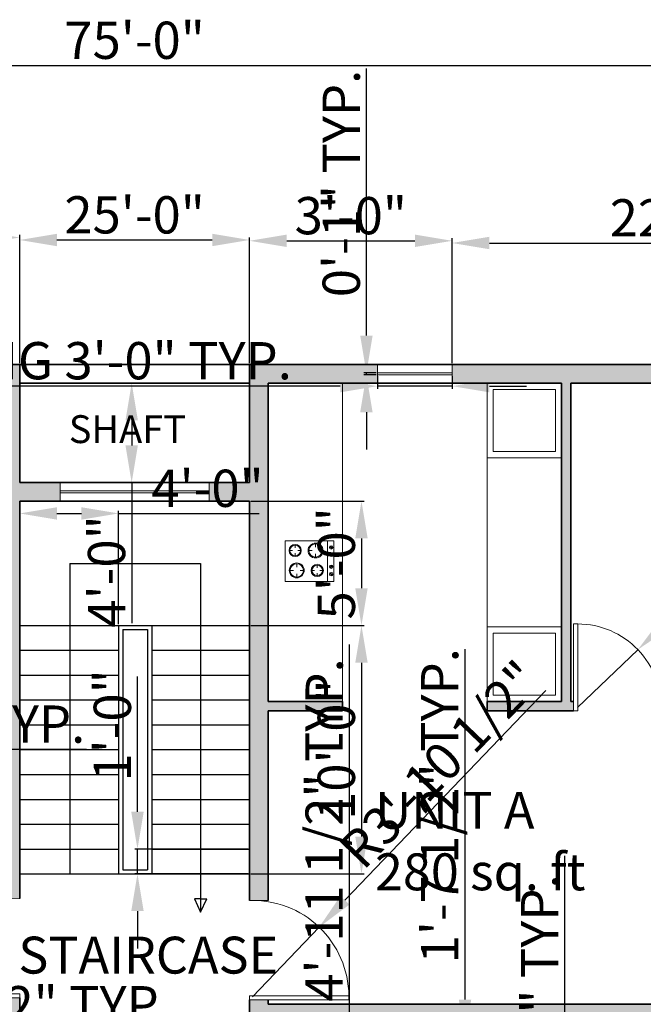
# Model space of a CAD drawing. Units: inches. Extents: x 2043 to 3177, y 1429 to 2563.
# Tile 13 of 14: x 2552 to 2853, y 1952 to 2428. Entities that reach past the tile are written whole.
import ezdxf

# ---------------------------------------------------------------- set-up
doc = ezdxf.new("R2010")
doc.units = ezdxf.units.IN
for name, color, linetype, lineweight in [('A-ANNO-DIMS', 2, 'Continuous', 13), ('A-AREA-IDEN', 7, 'Continuous', 18), ('A-DOOR', 3, 'Continuous', 18), ('A-EQPM', 8, 'Continuous', 18), ('A-FLOR-CASE', 8, 'Continuous', 18), ('A-FLOR-STRS', 7, 'Continuous', 25), ('A-GLAZ', 4, 'Continuous', 18), ('A-WALL', 7, 'Continuous', 35)]:
    doc.layers.add(name, color=color, linetype=linetype, lineweight=lineweight)
doc.layers.add('A-WALL-PATT', color=251, linetype='Continuous', lineweight=13, true_color=0x636466)
doc.styles.get("Standard").update_dxf_attribs({"font": 'arial.ttf'})
doc.dimstyles.new('ISO-25', dxfattribs={"dimtxt": 18, "dimasz": 18, "dimexe": 1.25, "dimexo": 0.625, "dimtad": 1, "dimlunit": 3, "dimtxsty": 'Standard', "dimcen": 2.5, "dimadec": 0, "dimazin": 0, "dimtfac": 1, "dimtmove": 0, "dimatfit": 3, "dimfxl": 1, "dimarcsym": 0})

# ---------------------------------------------------------------- blocks, each defined once
blk = doc.blocks.new('A$C16A60262')
at = {"linetype": 'ByBlock'}
for p, q in [((0, 600), (0, 0)), ((488, 600), (0, 600)), ((0, 600), (500, 600)), ((0, 600), (500, 600)), ((500, 520), (0, 520)), ((500, 600), (500, 0)), ((500, 600), (500, 0)), ((38, 374), (79, 374)), ((119, 456), (119, 415)), ((201, 374), (160, 374)), ((298, 395), (331, 395)), ((363, 460), (363, 427)), ((428, 395), (396, 395)), ((119, 293), (119, 334)), ((363, 330), (363, 362)), ((54, 124), (87, 124)), ((119, 189), (119, 156)), ((184, 124), (152, 124)), ((282, 144), (323, 144)), ((363, 225), (363, 185)), ((445, 144), (404, 144)), ((0, 0), (500, 0)), ((119, 59), (119, 91)), ((363, 63), (363, 103))]:
    blk.add_line(p, q, dxfattribs=at)
for p, q in [((66, 557), (87, 579)), ((72, 552), (66, 557)), ((93, 573), (72, 552)), ((87, 579), (93, 573)), ((158, 572), (163, 578)), ((179, 551), (158, 572)), ((163, 578), (184, 557)), ((184, 557), (179, 551)), ((305, 572), (311, 578)), ((326, 551), (305, 572)), ((311, 578), (332, 557)), ((332, 557), (326, 551)), ((396, 558), (417, 580)), ((402, 553), (396, 558)), ((423, 574), (402, 553)), ((417, 580), (423, 574))]:
    blk.add_line(p, q)
for centre in [(80, 566), (171, 566), (318, 566), (409, 566)]:
    blk.add_circle(centre, 20.6)
for centre, radius in [((119, 374), 91.3), ((119, 374), 81.3), ((363, 395), 75), ((363, 395), 65), ((119, 124), 75), ((119, 124), 65), ((363, 144), 91.3), ((363, 144), 81.3)]:
    blk.add_circle(centre, radius, dxfattribs=at)
blk = doc.blocks.new('*D13')
at = {"layer": 'A-ANNO-DIMS', "color": 0, "lineweight": -2, "transparency": 16777216}
for p, q in [((2453.87, 2262.02), (2453.87, 2324.03)), ((2471.87, 2322.78), (2533.74, 2322.78)), ((2551.74, 2262.02), (2551.74, 2324.03))]:
    blk.add_line(p, q, dxfattribs=at)
at = {"layer": 'A-ANNO-DIMS', "color": 0, "transparency": 16777216}
for points in [[(2471.87, 2325.78), (2471.87, 2319.78), (2453.87, 2322.78)], [(2533.74, 2325.78), (2533.74, 2319.78), (2551.74, 2322.78)]]:
    blk.add_solid(points, dxfattribs=at)
at = {"layer": 'Defpoints', "color": 0, "transparency": 16777216}
for p in [(2551.74, 2322.78), (2453.87, 2261.39), (2551.74, 2261.39)]:
    blk.add_point(p, dxfattribs=at)
at = {"layer": 'A-ANNO-DIMS', "color": 0, "transparency": 16777216, "insert": (2502.81, 2332.6), "char_height": 18, "attachment_point": 5}
blk.add_mtext('3\'-0"', dxfattribs=at)
blk = doc.blocks.new('*D14')
at = {"layer": 'A-ANNO-DIMS', "color": 0, "lineweight": -2, "transparency": 16777216}
for p, q in [((2551.74, 2262.02), (2551.74, 2322.83)), ((2569.74, 2321.58), (2644.74, 2321.58)), ((2662.74, 2262.02), (2662.74, 2322.83))]:
    blk.add_line(p, q, dxfattribs=at)
at = {"layer": 'A-ANNO-DIMS', "color": 0, "transparency": 16777216}
for points in [[(2569.74, 2324.58), (2569.74, 2318.58), (2551.74, 2321.58)], [(2644.74, 2324.58), (2644.74, 2318.58), (2662.74, 2321.58)]]:
    blk.add_solid(points, dxfattribs=at)
at = {"layer": 'Defpoints', "color": 0, "transparency": 16777216}
for p in [(2662.74, 2321.58), (2551.74, 2261.39), (2662.74, 2261.39)]:
    blk.add_point(p, dxfattribs=at)
at = {"layer": 'A-ANNO-DIMS', "color": 0, "transparency": 16777216, "insert": (2607.24, 2331.39), "char_height": 18, "attachment_point": 5}
blk.add_mtext('25\'-0"', dxfattribs=at)
blk = doc.blocks.new('*D15')
at = {"layer": 'A-ANNO-DIMS', "color": 0, "lineweight": -2, "transparency": 16777216}
for p, q in [((2662.74, 2262.02), (2662.74, 2322.43)), ((2680.74, 2321.18), (2742.62, 2321.18)), ((2760.62, 2262.02), (2760.62, 2322.43))]:
    blk.add_line(p, q, dxfattribs=at)
at = {"layer": 'A-ANNO-DIMS', "color": 0, "transparency": 16777216}
for points in [[(2680.74, 2324.18), (2680.74, 2318.18), (2662.74, 2321.18)], [(2742.62, 2324.18), (2742.62, 2318.18), (2760.62, 2321.18)]]:
    blk.add_solid(points, dxfattribs=at)
at = {"layer": 'Defpoints', "color": 0, "transparency": 16777216}
for p in [(2760.62, 2321.18), (2662.74, 2261.39), (2760.62, 2261.39)]:
    blk.add_point(p, dxfattribs=at)
at = {"layer": 'A-ANNO-DIMS', "color": 0, "transparency": 16777216, "insert": (2711.68, 2331), "char_height": 18, "attachment_point": 5}
blk.add_mtext('3\'-0"', dxfattribs=at)
blk = doc.blocks.new('*D16')
at = {"layer": 'A-ANNO-DIMS', "color": 0, "lineweight": -2, "transparency": 16777216}
for p, q in [((2760.62, 2262.02), (2760.62, 2321.37)), ((2980.74, 2262.02), (2980.74, 2321.37)), ((2778.62, 2320.12), (2962.74, 2320.12))]:
    blk.add_line(p, q, dxfattribs=at)
at = {"layer": 'A-ANNO-DIMS', "color": 0, "transparency": 16777216}
for points in [[(2778.62, 2323.12), (2778.62, 2317.12), (2760.62, 2320.12)], [(2962.74, 2323.12), (2962.74, 2317.12), (2980.74, 2320.12)]]:
    blk.add_solid(points, dxfattribs=at)
at = {"layer": 'Defpoints', "color": 0, "transparency": 16777216}
for p in [(2980.74, 2320.12), (2760.62, 2261.39), (2980.74, 2261.39)]:
    blk.add_point(p, dxfattribs=at)
at = {"layer": 'A-ANNO-DIMS', "color": 0, "transparency": 16777216, "insert": (2870.68, 2329.94), "char_height": 18, "attachment_point": 5}
blk.add_mtext('22\'-0"', dxfattribs=at)
blk = doc.blocks.new('*D30')
at = {"layer": 'A-ANNO-DIMS', "color": 0, "lineweight": -2, "transparency": 16777216}
for p, q in [((2233.74, 2262.02), (2233.74, 2407.15)), ((2980.74, 2262.02), (2980.74, 2407.15)), ((2251.74, 2405.9), (2962.74, 2405.9))]:
    blk.add_line(p, q, dxfattribs=at)
at = {"layer": 'A-ANNO-DIMS', "color": 0, "transparency": 16777216}
for points in [[(2251.74, 2408.9), (2251.74, 2402.9), (2233.74, 2405.9)], [(2962.74, 2408.9), (2962.74, 2402.9), (2980.74, 2405.9)]]:
    blk.add_solid(points, dxfattribs=at)
at = {"layer": 'Defpoints', "color": 0, "transparency": 16777216}
for p in [(2980.74, 2405.9), (2233.74, 2261.39), (2980.74, 2261.39)]:
    blk.add_point(p, dxfattribs=at)
at = {"layer": 'A-ANNO-DIMS', "color": 0, "transparency": 16777216, "insert": (2607.24, 2415.72), "char_height": 18, "attachment_point": 5}
blk.add_mtext('75\'-0"', dxfattribs=at)
blk = doc.blocks.new('CASEWORK-TWIN-END-BAYS')
for p, q in [((36, 153.75), (36, 0)), ((3, 150.75), (3, 120.75)), ((3, 150.75), (33, 150.75)), ((33, 150.75), (33, 120.75)), ((3, 120.75), (33, 120.75)), ((0, 117.75), (36, 117.75)), ((0, 36), (36, 36)), ((3, 33), (33, 33)), ((3, 33), (3, 3)), ((33, 33), (33, 3)), ((3, 3), (33, 3))]:
    blk.add_line(p, q)
blk = doc.blocks.new('GLAZING-36')
for p, q in [((0, 36), (0, 0)), ((1, 36), (1, 0))]:
    blk.add_line(p, q)
blk = doc.blocks.new('GLAZING-72')
for p, q in [((72, 1), (0, 1)), ((72, 0), (0, 0))]:
    blk.add_line(p, q)
blk = doc.blocks.new('*D41')
at = {"layer": 'A-ANNO-DIMS', "color": 0, "lineweight": -2, "transparency": 16777216}
for p, q in [((2711.06, 1791.23), (2711.06, 2126.25)), ((2702.73, 1791.23), (2712.31, 1791.23)), ((2711.06, 1749.52), (2711.06, 1773.23)), ((2702.73, 1731.52), (2712.31, 1731.52))]:
    blk.add_line(p, q, dxfattribs=at)
at = {"layer": 'A-ANNO-DIMS', "color": 0, "transparency": 16777216}
for points in [[(2708.06, 1773.23), (2714.06, 1773.23), (2711.06, 1791.23)], [(2708.06, 1749.52), (2714.06, 1749.52), (2711.06, 1731.52)]]:
    blk.add_solid(points, dxfattribs=at)
at = {"layer": 'Defpoints', "color": 0, "transparency": 16777216}
for p in [(2702.11, 1791.23), (2711.06, 1791.23), (2702.11, 1731.52)]:
    blk.add_point(p, dxfattribs=at)
at = {"layer": 'A-ANNO-DIMS', "color": 0, "transparency": 16777216, "insert": (2701.13, 1967.74), "char_height": 18, "attachment_point": 5, "rotation": 90}
blk.add_mtext('LOW TABLE 4\'-11 1/2" TYP.', dxfattribs=at)
blk = doc.blocks.new('*D49')
at = {"layer": 'A-ANNO-DIMS', "color": 0, "lineweight": -2, "transparency": 16777216}
for p, q in [((2724.62, 2255.77), (2724.62, 2249.74)), ((2760.62, 2255.77), (2760.62, 2249.74)), ((2706.62, 2250.99), (2460.58, 2250.99)), ((2760.62, 2250.99), (2724.62, 2250.99)), ((2778.62, 2250.99), (2796.62, 2250.99))]:
    blk.add_line(p, q, dxfattribs=at)
at = {"layer": 'A-ANNO-DIMS', "color": 0, "transparency": 16777216}
for points in [[(2706.62, 2253.99), (2706.62, 2247.99), (2724.62, 2250.99)], [(2778.62, 2253.99), (2778.62, 2247.99), (2760.62, 2250.99)]]:
    blk.add_solid(points, dxfattribs=at)
at = {"layer": 'Defpoints', "color": 0, "transparency": 16777216}
for p in [(2724.62, 2256.39), (2760.62, 2256.39), (2724.62, 2250.99)]:
    blk.add_point(p, dxfattribs=at)
at = {"layer": 'A-ANNO-DIMS', "color": 0, "transparency": 16777216, "insert": (2574.6, 2260.93), "char_height": 18, "attachment_point": 5}
blk.add_mtext('GLAZING 3\'-0" TYP.', dxfattribs=at)
blk = doc.blocks.new('*D50')
at = {"layer": 'A-ANNO-DIMS', "color": 0, "lineweight": -2, "transparency": 16777216}
for p, q in [((2719.22, 2275.39), (2719.22, 2404.36)), ((2723.99, 2257.39), (2717.97, 2257.39)), ((2723.99, 2256.39), (2717.97, 2256.39)), ((2719.22, 2256.39), (2719.22, 2257.39)), ((2719.22, 2238.39), (2719.22, 2220.39))]:
    blk.add_line(p, q, dxfattribs=at)
at = {"layer": 'A-ANNO-DIMS', "color": 0, "transparency": 16777216}
for points in [[(2716.22, 2275.39), (2722.22, 2275.39), (2719.22, 2257.39)], [(2716.22, 2238.39), (2722.22, 2238.39), (2719.22, 2256.39)]]:
    blk.add_solid(points, dxfattribs=at)
at = {"layer": 'Defpoints', "color": 0, "transparency": 16777216}
for p in [(2719.22, 2257.39), (2724.62, 2257.39), (2724.62, 2256.39)]:
    blk.add_point(p, dxfattribs=at)
at = {"layer": 'A-ANNO-DIMS', "color": 0, "transparency": 16777216, "insert": (2709.4, 2348.88), "char_height": 18, "attachment_point": 5, "rotation": 90}
blk.add_mtext('0\'-1" TYP.', dxfattribs=at)
blk = doc.blocks.new('*D57')
at = {"layer": 'A-ANNO-DIMS', "color": 0, "lineweight": -2, "transparency": 16777216}
for p, q in [((2309.03, 1935.24), (2309.03, 1941.18)), ((2344.46, 1935.24), (2344.46, 1941.18)), ((2291.03, 1939.93), (2273.03, 1939.93)), ((2309.03, 1939.93), (2344.46, 1939.93)), ((2362.46, 1939.93), (2629.01, 1939.93))]:
    blk.add_line(p, q, dxfattribs=at)
at = {"layer": 'A-ANNO-DIMS', "color": 0, "transparency": 16777216}
for points in [[(2291.03, 1942.93), (2291.03, 1936.93), (2309.03, 1939.93)], [(2362.46, 1942.93), (2362.46, 1936.93), (2344.46, 1939.93)]]:
    blk.add_solid(points, dxfattribs=at)
at = {"layer": 'Defpoints', "color": 0, "transparency": 16777216}
for p in [(2344.46, 1939.93), (2309.03, 1934.62), (2344.46, 1934.62)]:
    blk.add_point(p, dxfattribs=at)
at = {"layer": 'A-ANNO-DIMS', "color": 0, "transparency": 16777216, "insert": (2504.74, 1949.86), "char_height": 18, "attachment_point": 5}
blk.add_mtext('BASIN 2\'-11 1/2" TYP.', dxfattribs=at)
blk = doc.blocks.new('*D61')
at = {"layer": 'A-ANNO-DIMS', "color": 0, "lineweight": -2, "transparency": 16777216}
for p, q in [((2752.39, 1913.46), (2434.98, 1913.46)), ((2770.39, 1916.38), (2770.39, 1912.21)), ((2794.01, 1913.46), (2770.39, 1913.46)), ((2794.01, 1916.38), (2794.01, 1912.21)), ((2812.01, 1913.46), (2830.01, 1913.46))]:
    blk.add_line(p, q, dxfattribs=at)
at = {"layer": 'A-ANNO-DIMS', "color": 0, "transparency": 16777216}
for points in [[(2752.39, 1916.46), (2752.39, 1910.46), (2770.39, 1913.46)], [(2812.01, 1916.46), (2812.01, 1910.46), (2794.01, 1913.46)]]:
    blk.add_solid(points, dxfattribs=at)
at = {"layer": 'Defpoints', "color": 0, "transparency": 16777216}
for p in [(2770.39, 1917.01), (2794.01, 1917.01), (2770.39, 1913.46)]:
    blk.add_point(p, dxfattribs=at)
at = {"layer": 'A-ANNO-DIMS', "color": 0, "transparency": 16777216, "insert": (2584.68, 1923.4), "char_height": 18, "attachment_point": 5}
blk.add_mtext('COOKTOP 1\'-11 1/2" TYP.', dxfattribs=at)
blk = doc.blocks.new('*D62')
at = {"layer": 'A-ANNO-DIMS', "color": 0, "lineweight": -2, "transparency": 16777216}
for p, q in [((2766.85, 1954.69), (2766.85, 2123.91)), ((2769.77, 1936.69), (2765.6, 1936.69)), ((2766.85, 1917.01), (2766.85, 1936.69)), ((2769.77, 1917.01), (2765.6, 1917.01)), ((2766.85, 1899.01), (2766.85, 1881.01))]:
    blk.add_line(p, q, dxfattribs=at)
at = {"layer": 'A-ANNO-DIMS', "color": 0, "transparency": 16777216}
for points in [[(2763.85, 1954.69), (2769.85, 1954.69), (2766.85, 1936.69)], [(2763.85, 1899.01), (2769.85, 1899.01), (2766.85, 1917.01)]]:
    blk.add_solid(points, dxfattribs=at)
at = {"layer": 'Defpoints', "color": 0, "transparency": 16777216}
for p in [(2766.85, 1936.69), (2770.39, 1936.69), (2770.39, 1917.01)]:
    blk.add_point(p, dxfattribs=at)
at = {"layer": 'A-ANNO-DIMS', "color": 0, "transparency": 16777216, "insert": (2756.92, 2048.3), "char_height": 18, "attachment_point": 5, "rotation": 90}
blk.add_mtext('1\'-7 1/2" TYP.', dxfattribs=at)
blk = doc.blocks.new('*D64')
at = {"layer": 'A-ANNO-DIMS', "color": 0, "lineweight": -2, "transparency": 16777216}
for p, q in [((2400.99, 2098.02), (2400.99, 2074.33)), ((2436.99, 2098.02), (2436.99, 2074.33)), ((2382.99, 2075.58), (2364.99, 2075.58)), ((2400.99, 2075.58), (2436.99, 2075.58)), ((2454.99, 2075.58), (2583.95, 2075.58))]:
    blk.add_line(p, q, dxfattribs=at)
at = {"layer": 'A-ANNO-DIMS', "color": 0, "transparency": 16777216}
for points in [[(2382.99, 2078.58), (2382.99, 2072.58), (2400.99, 2075.58)], [(2454.99, 2078.58), (2454.99, 2072.58), (2436.99, 2075.58)]]:
    blk.add_solid(points, dxfattribs=at)
at = {"layer": 'Defpoints', "color": 0, "transparency": 16777216}
for p in [(2400.99, 2098.64), (2436.99, 2098.64), (2436.99, 2075.58)]:
    blk.add_point(p, dxfattribs=at)
at = {"layer": 'A-ANNO-DIMS', "color": 0, "transparency": 16777216, "insert": (2528.47, 2085.4), "char_height": 18, "attachment_point": 5}
blk.add_mtext('3\'-0" TYP.', dxfattribs=at)
blk = doc.blocks.new('*D65')
at = {"layer": 'A-ANNO-DIMS', "color": 0, "lineweight": -2, "transparency": 16777216}
for p, q in [((2815.14, 1739.39), (2815.14, 2024.17)), ((2801.37, 1739.39), (2816.39, 1739.39)), ((2815.14, 1661.39), (2815.14, 1721.39)), ((2801.37, 1643.39), (2816.39, 1643.39))]:
    blk.add_line(p, q, dxfattribs=at)
at = {"layer": 'A-ANNO-DIMS', "color": 0, "transparency": 16777216}
for points in [[(2812.14, 1721.39), (2818.14, 1721.39), (2815.14, 1739.39)], [(2812.14, 1661.39), (2818.14, 1661.39), (2815.14, 1643.39)]]:
    blk.add_solid(points, dxfattribs=at)
at = {"layer": 'Defpoints', "color": 0, "transparency": 16777216}
for p in [(2800.74, 1739.39), (2815.14, 1739.39), (2800.74, 1643.39)]:
    blk.add_point(p, dxfattribs=at)
at = {"layer": 'A-ANNO-DIMS', "color": 0, "transparency": 16777216, "insert": (2805.21, 1890.78), "char_height": 18, "attachment_point": 5, "rotation": 90}
blk.add_mtext('WARDROBE 8\'-0" TYP.', dxfattribs=at)
blk = doc.blocks.new('*D77')
at = {"layer": 'A-ANNO-DIMS', "color": 0, "lineweight": -2, "transparency": 16777216}
for p, q in [((2551.74, 2136.02), (2551.74, 2190.74)), ((2569.74, 2189.49), (2581.54, 2189.49)), ((2599.54, 2136.02), (2599.54, 2190.74)), ((2599.54, 2189.49), (2667.37, 2189.49))]:
    blk.add_line(p, q, dxfattribs=at)
at = {"layer": 'A-ANNO-DIMS', "color": 0, "transparency": 16777216}
for points in [[(2569.74, 2192.49), (2569.74, 2186.49), (2551.74, 2189.49)], [(2581.54, 2192.49), (2581.54, 2186.49), (2599.54, 2189.49)]]:
    blk.add_solid(points, dxfattribs=at)
at = {"layer": 'Defpoints', "color": 0, "transparency": 16777216}
for p in [(2599.54, 2189.49), (2551.74, 2135.39), (2599.54, 2135.39)]:
    blk.add_point(p, dxfattribs=at)
at = {"layer": 'A-ANNO-DIMS', "color": 0, "transparency": 16777216, "insert": (2642.46, 2199.31), "char_height": 18, "attachment_point": 5}
blk.add_mtext('4\'-0"', dxfattribs=at)
blk = doc.blocks.new('*D78')
at = {"layer": 'A-ANNO-DIMS', "color": 0, "lineweight": -2, "transparency": 16777216}
for p, q in [((2663.37, 2135.39), (2718.09, 2135.39)), ((2716.84, 2117.39), (2716.84, 2033.39)), ((2663.37, 2015.39), (2718.09, 2015.39))]:
    blk.add_line(p, q, dxfattribs=at)
at = {"layer": 'A-ANNO-DIMS', "color": 0, "transparency": 16777216}
for points in [[(2713.84, 2117.39), (2719.84, 2117.39), (2716.84, 2135.39)], [(2713.84, 2033.39), (2719.84, 2033.39), (2716.84, 2015.39)]]:
    blk.add_solid(points, dxfattribs=at)
at = {"layer": 'Defpoints', "color": 0, "transparency": 16777216}
for p in [(2662.74, 2135.39), (2662.74, 2015.39), (2716.84, 2015.39)]:
    blk.add_point(p, dxfattribs=at)
at = {"layer": 'A-ANNO-DIMS', "color": 0, "transparency": 16777216, "insert": (2707.03, 2075.39), "char_height": 18, "attachment_point": 5, "rotation": 90}
blk.add_mtext('10\'-0"', dxfattribs=at)
blk = doc.blocks.new('*D79')
at = {"layer": 'A-ANNO-DIMS', "color": 0, "lineweight": -2, "transparency": 16777216}
for p, q in [((2663.37, 2195.39), (2718.09, 2195.39)), ((2716.84, 2177.39), (2716.84, 2153.39)), ((2663.37, 2135.39), (2718.09, 2135.39))]:
    blk.add_line(p, q, dxfattribs=at)
at = {"layer": 'A-ANNO-DIMS', "color": 0, "transparency": 16777216}
for points in [[(2713.84, 2177.39), (2719.84, 2177.39), (2716.84, 2195.39)], [(2713.84, 2153.39), (2719.84, 2153.39), (2716.84, 2135.39)]]:
    blk.add_solid(points, dxfattribs=at)
at = {"layer": 'Defpoints', "color": 0, "transparency": 16777216}
for p in [(2662.74, 2195.39), (2662.74, 2135.39), (2716.84, 2135.39)]:
    blk.add_point(p, dxfattribs=at)
at = {"layer": 'A-ANNO-DIMS', "color": 0, "transparency": 16777216, "insert": (2707.03, 2165.39), "char_height": 18, "attachment_point": 5, "rotation": 90}
blk.add_mtext('5\'-0"', dxfattribs=at)
blk = doc.blocks.new('*D80')
at = {"layer": 'A-ANNO-DIMS', "color": 0, "lineweight": -2, "transparency": 16777216}
for p, q in [((2552.37, 2252.39), (2607.09, 2252.39)), ((2605.84, 2234.39), (2605.84, 2222.39)), ((2552.37, 2204.39), (2607.09, 2204.39)), ((2605.84, 2204.39), (2605.84, 2136.57))]:
    blk.add_line(p, q, dxfattribs=at)
at = {"layer": 'A-ANNO-DIMS', "color": 0, "transparency": 16777216}
for points in [[(2602.84, 2234.39), (2608.84, 2234.39), (2605.84, 2252.39)], [(2602.84, 2222.39), (2608.84, 2222.39), (2605.84, 2204.39)]]:
    blk.add_solid(points, dxfattribs=at)
at = {"layer": 'Defpoints', "color": 0, "transparency": 16777216}
for p in [(2551.74, 2252.39), (2551.74, 2204.39), (2605.84, 2204.39)]:
    blk.add_point(p, dxfattribs=at)
at = {"layer": 'A-ANNO-DIMS', "color": 0, "transparency": 16777216, "insert": (2596.03, 2161.48), "char_height": 18, "attachment_point": 5, "rotation": 90}
blk.add_mtext('4\'-0"', dxfattribs=at)
blk = doc.blocks.new('*D82')
at = {"layer": 'A-ANNO-DIMS', "color": 0, "lineweight": -2, "transparency": 16777216}
for p, q in [((2608.64, 2045.39), (2608.64, 2110.8)), ((2662.12, 2027.39), (2607.39, 2027.39)), ((2608.64, 2015.39), (2608.64, 2027.39)), ((2662.12, 2015.39), (2607.39, 2015.39)), ((2608.64, 1997.39), (2608.64, 1979.39))]:
    blk.add_line(p, q, dxfattribs=at)
at = {"layer": 'A-ANNO-DIMS', "color": 0, "transparency": 16777216}
for points in [[(2605.64, 2045.39), (2611.64, 2045.39), (2608.64, 2027.39)], [(2605.64, 1997.39), (2611.64, 1997.39), (2608.64, 2015.39)]]:
    blk.add_solid(points, dxfattribs=at)
at = {"layer": 'Defpoints', "color": 0, "transparency": 16777216}
for p in [(2608.64, 2027.39), (2662.74, 2027.39), (2662.74, 2015.39)]:
    blk.add_point(p, dxfattribs=at)
at = {"layer": 'A-ANNO-DIMS', "color": 0, "transparency": 16777216, "insert": (2598.83, 2087.1), "char_height": 18, "attachment_point": 5, "rotation": 90}
blk.add_mtext('1\'-0"', dxfattribs=at)
blk = doc.blocks.new('*D87')
at = {"layer": 'A-ANNO-DIMS', "color": 0, "lineweight": -2, "transparency": 16777216}
for p, q in [((2805.9, 2103.9), (2708.86, 2002.64)), ((2664.2, 1956.04), (2696.41, 1989.65))]:
    blk.add_line(p, q, dxfattribs=at)
at = {"layer": 'A-ANNO-DIMS', "color": 0, "transparency": 16777216}
blk.add_solid([(2706.69, 2004.72), (2711.03, 2000.57), (2696.41, 1989.65)], dxfattribs=at)
at = {"layer": 'Defpoints', "color": 0, "transparency": 16777216}
for p in [(2696.41, 1989.65), (2664.2, 1956.04)]:
    blk.add_point(p, dxfattribs=at)
at = {"layer": 'A-ANNO-DIMS', "color": 0, "transparency": 16777216, "insert": (2756.43, 2066.65), "char_height": 18, "attachment_point": 5, "rotation": 46.219}
blk.add_mtext('R3\'-10 1/2"', dxfattribs=at)
blk = doc.blocks.new('*D90')
at = {"layer": 'A-ANNO-DIMS', "color": 0, "lineweight": -2, "transparency": 16777216}
for p, q in [((2954.57, 2223.44), (2863.34, 2136.14)), ((2821.19, 2095.8), (2850.33, 2123.69))]:
    blk.add_line(p, q, dxfattribs=at)
at = {"layer": 'A-ANNO-DIMS', "color": 0, "transparency": 16777216}
blk.add_solid([(2861.26, 2138.31), (2865.41, 2133.97), (2850.33, 2123.69)], dxfattribs=at)
at = {"layer": 'Defpoints', "color": 0, "transparency": 16777216}
for p in [(2850.33, 2123.69), (2821.19, 2095.8)]:
    blk.add_point(p, dxfattribs=at)
at = {"layer": 'A-ANNO-DIMS', "color": 0, "transparency": 16777216, "insert": (2908.58, 2193.19), "char_height": 18, "attachment_point": 5, "rotation": 43.7398}
blk.add_mtext('R3\'-4 1/2"', dxfattribs=at)

msp = doc.modelspace()

# ---------------------------------------------------------------- hatches: boundary and pattern name
at = {"layer": 'A-WALL-PATT'}
h = msp.add_hatch(color=256, dxfattribs=at)
h.dxf.hatch_style = 1
h.paths.add_polyline_path([(2283.62, 2261.393), (2233.745, 2261.393), (2233.745, 2029.268), (2242.745, 2029.268), (2242.745, 2070.143), (2348.495, 2070.143), (2348.495, 2063.887), (2352.995, 2063.887), (2352.995, 2094.143), (2353.364, 2094.143, -0.017175), (2353.364, 2096.932), (2353.364, 2098.643), (2348.495, 2098.643), (2348.495, 2096.393), (2348.495, 2074.643), (2242.745, 2074.643), (2242.745, 2252.393), (2283.62, 2252.393)])
h.paths.add_polyline_path([(2453.87, 2261.393), (2355.62, 2261.393), (2355.62, 2252.393), (2396.495, 2252.393), (2396.495, 2098.643), (2395.364, 2098.643), (2395.364, 2094.143), (2436.995, 2094.143), (2436.995, 2098.643), (2400.995, 2098.643), (2400.995, 2252.393), (2453.87, 2252.393)])
h.paths.add_polyline_path([(2551.745, 2261.393), (2489.87, 2261.393), (2489.87, 2252.393), (2542.745, 2252.393), (2542.745, 2098.643), (2506.745, 2098.643), (2506.745, 2094.143), (2542.745, 2094.143), (2542.745, 2003.513), (2549.809, 2003.513, -0.0102854), (2551.745, 2003.513), (2551.745, 2195.393), (2571.245, 2195.393), (2571.245, 2204.393), (2551.745, 2204.393)])
h.paths.add_polyline_path([(2724.62, 2261.393), (2662.745, 2261.393), (2662.745, 2204.393), (2643.245, 2204.393), (2643.245, 2195.393), (2662.745, 2195.393), (2662.745, 2002.566, -0.0156152), (2665.651, 2002.566), (2671.745, 2002.566), (2671.745, 2094.143), (2707.745, 2094.143), (2707.745, 2098.643), (2671.745, 2098.643), (2671.745, 2252.393), (2724.62, 2252.393)])
h.paths.add_polyline_path([(2858.87, 2261.393), (2760.62, 2261.393), (2760.62, 2252.393), (2813.495, 2252.393), (2813.495, 2098.643), (2777.495, 2098.643), (2777.495, 2094.143), (2819.302, 2094.143), (2819.302, 2098.643), (2817.995, 2098.643), (2817.995, 2252.393), (2858.87, 2252.393)])
h.paths.add_polyline_path([(2980.745, 2261.393), (2930.87, 2261.393), (2930.87, 2252.393), (2971.745, 2252.393), (2971.745, 2074.643), (2865.995, 2074.643), (2865.995, 2098.643), (2861.429, 2098.643, -0.0279128), (2861.495, 2094.143), (2861.495, 2063.254), (2865.995, 2063.254), (2865.995, 2070.143), (2971.745, 2070.143), (2971.745, 2029.268), (2980.745, 2029.268)])
h.paths.add_polyline_path([(2980.745, 1993.268), (2971.745, 1993.268), (2971.745, 1952.393), (2865.995, 1952.393), (2865.995, 2027.254), (2865.688, 2027.254, -0.0309542), (2861.495, 2027.254), (2861.495, 1952.393), (2671.745, 1952.393), (2671.745, 1954.566), (2662.745, 1954.566), (2662.745, 1883.393), (2661.473, 1883.393, -0.012912), (2661.473, 1880.977), (2661.473, 1874.393), (2671.745, 1874.393), (2671.745, 1943.393), (2861.495, 1943.393), (2861.495, 1903.412, -0.0351753), (2865.995, 1903.659), (2865.995, 1943.393), (2971.745, 1943.393), (2971.745, 1922.018), (2980.745, 1922.018)])
h.paths.add_polyline_path([(2980.745, 1886.018), (2971.745, 1886.018), (2971.745, 1864.643), (2865.995, 1864.643), (2865.995, 1867.412), (2861.495, 1867.412), (2861.495, 1840.643), (2828.844, 1840.643, -0.0159075), (2828.844, 1837.684), (2828.844, 1836.143), (2865.995, 1836.143), (2865.995, 1860.143), (2971.745, 1860.143), (2971.745, 1643.393), (2910.245, 1643.393), (2910.245, 1634.393), (2980.745, 1634.393)])
h.paths.add_polyline_path([(2776.745, 1836.143), (2780.844, 1836.143), (2780.844, 1840.643), (2772.245, 1840.643), (2772.245, 1679.393), (2760.995, 1679.393), (2760.995, 1670.393), (2767.745, 1670.393), (2767.745, 1634.393), (2838.245, 1634.393), (2838.245, 1643.393), (2776.745, 1643.393)])
h.paths.add_polyline_path([(2736.995, 1679.393), (2727.995, 1679.393), (2727.995, 1670.393), (2736.995, 1670.393)])
h.paths.add_polyline_path([(2667.995, 1679.393), (2611.745, 1679.393), (2611.745, 1874.393), (2613.473, 1874.393), (2613.473, 1883.393), (2600.336, 1883.393), (2600.336, 1874.393), (2602.745, 1874.393), (2602.745, 1679.393), (2546.495, 1679.393), (2546.495, 1670.393), (2667.995, 1670.393)])
h.paths.add_polyline_path([(2486.495, 1679.393), (2477.495, 1679.393), (2477.495, 1670.393), (2486.495, 1670.393)])
h.paths.add_polyline_path([(2453.495, 1679.393), (2442.245, 1679.393), (2442.245, 1839.893), (2427.654, 1839.893), (2427.654, 1835.393), (2437.745, 1835.393), (2437.745, 1643.393), (2376.245, 1643.393), (2376.245, 1634.393), (2446.745, 1634.393), (2446.745, 1670.393), (2453.495, 1670.393)])
h.paths.add_polyline_path([(2304.245, 1643.393), (2242.745, 1643.393), (2242.745, 1857.143), (2348.495, 1857.143), (2348.495, 1835.393), (2352.995, 1835.393), (2379.654, 1835.393), (2379.654, 1837.073, -0.0151369), (2379.654, 1839.893), (2352.995, 1839.893), (2352.995, 1867.394), (2348.495, 1867.394), (2348.495, 1861.643), (2242.745, 1861.643), (2242.745, 1884.518), (2233.745, 1884.518), (2233.745, 1634.393), (2304.245, 1634.393)])
h.paths.add_polyline_path([(2551.745, 1955.513), (2542.745, 1955.513), (2542.745, 1952.393), (2352.995, 1952.393), (2352.995, 2027.887, -0.0208198), (2350.117, 2027.887), (2348.495, 2027.887), (2348.495, 1952.393), (2242.745, 1952.393), (2242.745, 1993.268), (2233.745, 1993.268), (2233.745, 1943.393), (2233.745, 1920.518), (2242.745, 1920.518), (2242.745, 1943.393), (2348.495, 1943.393), (2348.495, 1903.394), (2352.995, 1903.394), (2352.995, 1943.393), (2542.745, 1943.393), (2542.745, 1874.393), (2552.336, 1874.393), (2552.336, 1880.494, -0.0155728), (2552.336, 1883.393), (2551.745, 1883.393)])

# ---------------------------------------------------------------- linework, layer by layer
at = {"layer": 'A-DOOR'}
for p, q in [((2819.302, 2094.143), (2819.302, 2136.143)), ((2819.302, 2136.143), (2821.302, 2136.143)), ((2821.302, 2136.143), (2821.302, 2094.143)), ((2819.302, 2098.643), (2819.302, 2094.143)), ((2821.302, 2094.143), (2819.302, 2094.143)), ((2671.745, 2002.566), (2662.745, 2002.566)), ((2503.745, 1957.513), (2551.745, 1957.513)), ((2551.745, 1955.513), (2503.745, 1955.513)), ((2542.745, 1955.513), (2551.745, 1955.513)), ((2551.745, 1957.513), (2551.745, 1955.513)), ((2710.745, 1956.566), (2662.745, 1956.566)), ((2662.745, 1956.566), (2662.745, 1954.566)), ((2710.745, 1954.566), (2710.745, 1956.566)), ((2671.745, 1954.566), (2662.745, 1954.566)), ((2662.745, 1954.566), (2710.745, 1954.566))]:
    msp.add_line(p, q, dxfattribs=at)
for centre, radius, start, end in [((2821.189, 2095.804), 40.34, 357.64105, 89.83908), ((2550.777, 1956.479), 47.044, 88.82142, 178.74083), ((2664.198, 1956.04), 46.55, 0.64852, 91.78923)]:
    msp.add_arc(centre, radius, start, end, dxfattribs=at)
at = {"layer": 'A-FLOR-CASE'}
msp.add_line((2707.745, 2098.643), (2707.745, 2252.393), dxfattribs=at)
at = {"layer": 'A-FLOR-STRS'}
for p, q in [((2575.945, 2165.393), (2639.145, 2165.393)), ((2575.945, 2165.393), (2575.945, 2015.393)), ((2639.145, 2165.393), (2639.145, 1996.966)), ((2551.745, 2135.393), (2662.745, 2135.393)), ((2599.545, 2135.393), (2599.545, 2015.393)), ((2601.545, 2133.393), (2601.545, 2017.393)), ((2601.545, 2133.393), (2613.545, 2133.393)), ((2613.545, 2133.393), (2613.545, 2017.393)), ((2615.545, 2135.393), (2615.545, 2015.393)), ((2551.745, 2123.393), (2599.545, 2123.393)), ((2615.545, 2123.393), (2662.745, 2123.393)), ((2551.745, 2111.393), (2599.545, 2111.393)), ((2615.545, 2111.393), (2662.745, 2111.393)), ((2551.745, 2099.393), (2599.545, 2099.393)), ((2615.545, 2099.393), (2662.745, 2099.393)), ((2551.745, 2087.393), (2599.545, 2087.393)), ((2615.545, 2087.393), (2662.745, 2087.393)), ((2551.745, 2075.393), (2599.545, 2075.393)), ((2615.545, 2075.393), (2662.745, 2075.393)), ((2551.745, 2063.393), (2599.545, 2063.393)), ((2615.545, 2063.393), (2662.745, 2063.393)), ((2551.745, 2051.393), (2599.545, 2051.393)), ((2615.545, 2051.393), (2662.745, 2051.393)), ((2551.745, 2039.393), (2599.545, 2039.393)), ((2615.545, 2039.393), (2662.745, 2039.393)), ((2551.745, 2027.393), (2599.545, 2027.393)), ((2615.545, 2027.393), (2662.745, 2027.393)), ((2601.545, 2017.393), (2613.545, 2017.393)), ((2551.745, 2015.393), (2662.745, 2015.393)), ((2639.145, 2003.337), (2636.145, 2003.337)), ((2636.145, 2003.337), (2639.145, 1996.966)), ((2639.145, 2003.337), (2642.145, 2003.337)), ((2639.145, 1996.966), (2642.145, 2003.337))]:
    msp.add_line(p, q, dxfattribs=at)
at = {"layer": 'A-GLAZ'}
for p, q in [((2724.62, 2252.393), (2724.62, 2261.393)), ((2760.62, 2252.393), (2760.62, 2261.393)), ((2571.245, 2195.393), (2571.245, 2204.393)), ((2643.245, 2195.393), (2643.245, 2204.393))]:
    msp.add_line(p, q, dxfattribs=at)
at = {"layer": 'A-WALL'}
for p, q in [((2233.745, 2261.393), (2551.745, 2261.393)), ((2551.745, 2261.393), (2551.745, 2204.393)), ((2551.745, 2261.393), (2662.745, 2261.393)), ((2662.745, 2261.393), (2980.745, 2261.393)), ((2662.745, 2204.393), (2662.745, 2261.393)), ((2551.745, 2252.393), (2662.745, 2252.393)), ((2671.745, 2252.393), (2813.495, 2252.393)), ((2671.745, 2098.643), (2671.745, 2252.393)), ((2813.495, 2098.643), (2813.495, 2252.393)), ((2817.995, 2098.643), (2817.995, 2252.393)), ((2817.995, 2252.393), (2971.745, 2252.393)), ((2551.745, 2204.393), (2662.745, 2204.393)), ((2551.745, 2195.393), (2662.745, 2195.393)), ((2551.745, 2195.393), (2551.745, 2003.513)), ((2662.745, 2002.566), (2662.745, 2195.393)), ((2671.745, 2098.643), (2707.745, 2098.643)), ((2707.745, 2098.643), (2707.745, 2094.143)), ((2777.495, 2098.643), (2777.495, 2094.143)), ((2777.495, 2098.643), (2813.495, 2098.643)), ((2817.995, 2098.643), (2819.302, 2098.643)), ((2671.745, 2094.143), (2707.745, 2094.143)), ((2671.745, 2002.566), (2671.745, 2094.143)), ((2777.495, 2094.143), (2819.302, 2094.143)), ((2551.745, 1955.513), (2551.745, 1883.393)), ((2662.745, 1883.393), (2662.745, 1954.566)), ((2671.745, 1952.393), (2671.745, 1954.566)), ((2861.495, 1952.393), (2671.745, 1952.393))]:
    msp.add_line(p, q, dxfattribs=at)

# ---------------------------------------------------------------- block references
at = {"layer": 'A-EQPM', "xscale": 0.0393700787401575, "yscale": 0.0393700787401575, "zscale": 0.0393700787401575, "rotation": 269.9999999999978}
msp.add_blockref('A$C16A60262', (2679.911, 2176.258), dxfattribs=at)
at = {"layer": 'A-FLOR-CASE', "rotation": 180}
msp.add_blockref('CASEWORK-TWIN-END-BAYS', (2813.494, 2252.394), dxfattribs=at)
at = {"layer": 'A-GLAZ', "rotation": 90.00000000000006}
msp.add_blockref('GLAZING-36', (2760.62, 2256.394), dxfattribs=at)
at = {"layer": 'A-GLAZ'}
msp.add_blockref('GLAZING-72', (2571.245, 2199.393), dxfattribs=at)

# ---------------------------------------------------------------- texts
at = {"layer": 'A-AREA-IDEN', "attachment_point": 1}
for s, width, gutter_width, insert, char_height in [('SHAFT', 381.44992, 67.303, (2575.473, 2236.941), 13.4607), ('UNIT A \\P280 sq. ft', 505.18079, 89.135, (2723.358, 2055.009), 17.8269), ('STAIRCASE', 505.18079, 89.135, (2551.094, 1985.064), 17.8269)]:
    msp.add_mtext_dynamic_manual_height_columns(s, width=width, gutter_width=gutter_width, heights=[0], dxfattribs=dict(at, insert=insert, char_height=char_height))

# ---------------------------------------------------------------- dimensions: what is measured, and where the dimension line sits
at = {"layer": 'A-ANNO-DIMS'}
for base, p1, p2, text, override, picture, middle in [((2980.745, 2405.904), (2233.745, 2261.393), (2980.745, 2261.393), '75\'-0"', {"dimclrd": 0, "dimclre": 0, "dimclrt": 0}, '*D30', (2607.245, 2415.72)), ((2551.745, 2322.782), (2453.87, 2261.393), (2551.745, 2261.393), '3\'-0"', {"dimclrd": 0, "dimclre": 0, "dimclrt": 0}, '*D13', (2502.807, 2332.603)), ((2662.745, 2321.577), (2551.745, 2261.393), (2662.745, 2261.393), '25\'-0"', {"dimclrd": 0, "dimclre": 0, "dimclrt": 0}, '*D14', (2607.245, 2331.392)), ((2760.62, 2321.181), (2662.745, 2261.393), (2760.62, 2261.393), '3\'-0"', {"dimclrd": 0, "dimclre": 0, "dimclrt": 0}, '*D15', (2711.682, 2331.002)), ((2980.745, 2320.123), (2760.62, 2261.393), (2980.745, 2261.393), '22\'-0"', {"dimclrd": 0, "dimclre": 0, "dimclrt": 0}, '*D16', (2870.682, 2329.938)), ((2436.995, 2075.581), (2400.995, 2098.643), (2436.995, 2098.643), '<> TYP.', {"dimdec": 1, "dimlfac": 1, "dimrnd": 0, "dimzin": 1, "dimdsep": 46, "dimlunit": 4, "dimfrac": 2}, '*D64', (2528.473, 2085.402)), ((2344.462, 1939.932), (2309.031, 1934.617), (2344.462, 1934.617), 'BASIN <> TYP.', {"dimdec": 1, "dimlfac": 1, "dimrnd": 0, "dimzin": 1, "dimdsep": 46, "dimlunit": 4, "dimfrac": 2}, '*D57', (2504.735, 1949.864))]:
    dim = msp.add_linear_dim(base=base, p1=p1, p2=p2, text=text, dimstyle='ISO-25', override=override, dxfattribs=at)
    dim.commit()
    dim.dimension.update_dxf_attribs({"geometry": picture, "text_midpoint": middle})
for base, p1, p2, angle, text, picture, middle in [((2719.22, 2257.393), (2724.62, 2256.393), (2724.62, 2257.393), 90, '<> TYP.', '*D50', (2709.404, 2348.878)), ((2724.62, 2250.993), (2760.62, 2256.393), (2724.62, 2256.393), 180, 'GLAZING <> TYP.', '*D49', (2574.598, 2260.931)), ((2711.065, 1791.234), (2702.108, 1731.521), (2702.108, 1791.234), 90, 'LOW TABLE <> TYP.', '*D41', (2701.127, 1967.74)), ((2766.849, 1936.692), (2770.393, 1917.007), (2770.393, 1936.692), 90, '<> TYP.', '*D62', (2756.918, 2048.301)), ((2815.145, 1739.393), (2800.745, 1643.393), (2800.745, 1739.393), 90, 'WARDROBE <> TYP.', '*D65', (2805.206, 1890.784)), ((2770.393, 1913.464), (2794.015, 1917.007), (2770.393, 1917.007), 180, 'COOKTOP <> TYP.', '*D61', (2584.685, 1923.402))]:
    dim = msp.add_linear_dim(base=base, p1=p1, p2=p2, angle=angle, text=text, dimstyle='ISO-25', override={"dimdec": 1, "dimlfac": 1, "dimrnd": 0, "dimzin": 1, "dimdsep": 46, "dimlunit": 4, "dimfrac": 2}, dxfattribs=at)
    dim.commit()
    dim.dimension.update_dxf_attribs({"geometry": picture, "text_midpoint": middle})
for base, p1, p2, angle, picture, middle in [((2605.845, 2204.393), (2551.745, 2252.393), (2551.745, 2204.393), 270, '*D80', (2596.029, 2161.482)), ((2716.845, 2135.393), (2662.745, 2195.393), (2662.745, 2135.393), 270, '*D79', (2707.029, 2165.393)), ((2716.845, 2015.393), (2662.745, 2135.393), (2662.745, 2015.393), 270, '*D78', (2707.029, 2075.393)), ((2608.645, 2027.393), (2662.745, 2015.393), (2662.745, 2027.393), 90, '*D82', (2598.829, 2087.095))]:
    dim = msp.add_linear_dim(base=base, p1=p1, p2=p2, angle=angle, dimstyle='ISO-25', override={"dimdec": 1, "dimlfac": 1, "dimrnd": 0, "dimzin": 1, "dimdsep": 46, "dimlunit": 4, "dimfrac": 2}, dxfattribs=at)
    dim.commit()
    dim.dimension.update_dxf_attribs({"geometry": picture, "text_midpoint": middle})
for center, mpoint, picture, middle in [((2821.189, 2095.804), (2850.334, 2123.694), '*D90', (2908.584, 2193.191)), ((2664.198, 1956.04), (2696.406, 1989.648), '*D87', (2756.433, 2066.648))]:
    dim = msp.add_radius_dim(center=center, mpoint=mpoint, dimstyle='ISO-25', override={"dimdec": 1, "dimlfac": 1, "dimrnd": 0, "dimzin": 1, "dimdsep": 46, "dimlunit": 4, "dimfrac": 2}, dxfattribs=at)
    dim.commit()
    dim.dimension.update_dxf_attribs({"geometry": picture, "text_midpoint": middle})
dim = msp.add_linear_dim(base=(2599.545, 2189.493), p1=(2551.745, 2135.393), p2=(2599.545, 2135.393), dimstyle='ISO-25', override={"dimdec": 1, "dimlfac": 1, "dimrnd": 0, "dimzin": 1, "dimdsep": 46, "dimlunit": 4, "dimfrac": 2}, dxfattribs=at)
dim.commit()
dim.dimension.update_dxf_attribs({"geometry": '*D77', "text_midpoint": (2642.456, 2199.309)})

doc.saveas('drawing.dxf')
